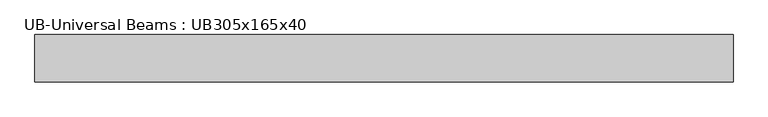
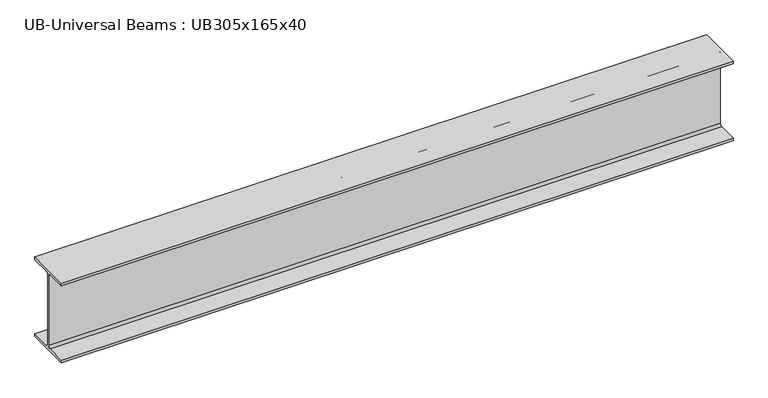
"""IFC4 building model written with IfcOpenShell, lengths in millimetres: beam geometry, UB-Universal Beams : UB305x165x40."""

from ifc_helpers import new_model, si_unit, point, frame, frame_2d, origin, place, context, project, spatial, polyline, circle_curve, trimmed, segment, composite_curve, outline, extrude, source, transform, mapped, element, save


def ub_universal_beams_ub305x165x40_b9dd2748(model_context):
    return source(origin(), model_context, "Body", "SweptSolid", [
        extrude(outline(composite_curve([segment(polyline([(82.5, -141.5), (82.5, -151.7), (-82.5, -151.7), (-82.5, -141.5), (-11.9, -141.5)]), True, "CONTINUOUS"), segment(trimmed(circle_curve(frame_2d((-11.9, -132.6)), 8.9), [point((-11.9, -141.5))], [point((-3.0, -132.6))], True, "CARTESIAN"), True, "CONTINUOUS"), segment(polyline([(-3.0, -132.6), (-3.0, 132.6)]), True, "CONTINUOUS"), segment(trimmed(circle_curve(frame_2d((-11.9, 132.6)), 8.9), [point((-3.0, 132.6))], [point((-11.9, 141.5))], True, "CARTESIAN"), True, "CONTINUOUS"), segment(polyline([(-11.9, 141.5), (-82.5, 141.5), (-82.5, 151.7), (82.5, 151.7), (82.5, 141.5), (11.9, 141.5)]), True, "CONTINUOUS"), segment(trimmed(circle_curve(frame_2d((11.9, 132.6)), 8.9), [point((11.9, 141.5))], [point((3.0, 132.6))], True, "CARTESIAN"), True, "CONTINUOUS"), segment(polyline([(3.0, 132.6), (3.0, -132.6)]), True, "CONTINUOUS"), segment(trimmed(circle_curve(frame_2d((11.9, -132.6)), 8.9), [point((3.0, -132.6))], [point((11.9, -141.5))], True, "CARTESIAN"), True, "CONTINUOUS"), segment(polyline([(11.9, -141.5), (82.5, -141.5)]), True, "CONTINUOUS")], self_intersect=False)), frame((-1256.15, 0.0, 0.0), z_axis=(1.0, 0.0, 0.0), x_axis=(0.0, 1.0, 0.0)), (0.0, 0.0, 1.0), 2422.0),
    ])


if __name__ == "__main__":
    model = new_model("IFC4")
    model_context = context("Model", 3, world=origin())
    ifc_project = project(units=[si_unit("LENGTHUNIT", "METRE", prefix="MILLI")], contexts=[model_context])
    site = spatial("IfcSite", under=ifc_project)
    building = spatial("IfcBuilding", under=site)
    placement = place(None, origin())
    ub_universal_beams_ub305x165x40_shape = ub_universal_beams_ub305x165x40_b9dd2748(model_context)
    element("IfcBeam", 1, ObjectType="UB-Universal Beams : UB305x165x40", at=placement, inside=building, context=model_context, shape_type="MappedRepresentation", body=[
        mapped(ub_universal_beams_ub305x165x40_shape, transform((0.0, 0.0, 0.0), x_axis=(1.0, 0.0, 0.0), y_axis=(0.0, 1.0, 0.0), z_axis=(0.0, 0.0, 1.0))),
    ])
    save(model, "model.ifc")

# Revit data of these elements
# Type "UB-Universal Beams : UB305x165x40"
#   Section Name Key = "UB305X165X40"
#   Width = 16.5 cm
#   Web Thickness = 0.6 cm
#   Web Fillet = 0.89 cm
#   Warping Constant = 164000.0 cm⁶
#   Torsional Moment of Inertia = 14.70 cm⁴
#   Section Area = 51.3 cm²
#   Plastic Modulus weak axis = 142.0 cm³
#   Plastic Modulus strong axis = 623.0 cm³
#   Nominal Weight = 40.2999 kgf/m
#   Moment of Inertia weak axis = 764.00 cm⁴
#   Moment of Inertia strong axis = 8503.00 cm⁴
#   Height = 30.34 cm
#   Flange Thickness = 1.02 cm
#   Elastic Modulus weak axis = 92.6 cm³
#   Elastic Modulus strong axis = 560.0 cm³
#   Centroid Vertical = 15.17 cm
#   Centroid Horizontal = 8.25 cm
#   Bolt Spacing = 9.0 cm
#   Length [instance default] = 1500 mm
#   Structural Material [instance default] = Metal - Steel 43-275
#   Type Comments = ""
#   Assembly Code = ""
# Element 1 (IfcBeam, "UB-Universal Beams : UB305x165x40")
#   Materials on its faces: "Metal - Steel 43-275"
# Materials
#   "Metal - Steel 43-275": class "Metal", colour RGB 247 247 247, transparency 0, Cost = 0
